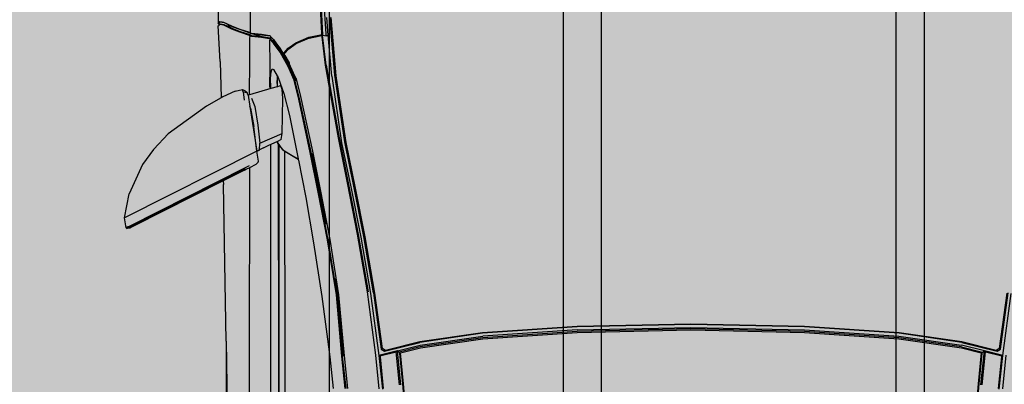
# Model space of a CAD drawing. Units: inches. Extents: x 1884 to 2398, y 474 to 1488.
# Tile 25 of 39: x 2275 to 2348, y 672 to 699. Entities that reach past the tile are written whole.
import ezdxf

# ---------------------------------------------------------------- set-up
doc = ezdxf.new("R2010")
doc.units = ezdxf.units.IN
doc.header["$MEASUREMENT"] = 0
doc.layers.get('0').update_dxf_attribs({"color": 250})
doc.layers.add('A-ANNO-DIMS', color=2, linetype='Continuous', lineweight=18)
doc.layers.add('C-VEHI', color=8, linetype='Continuous', lineweight=18)
doc.layers.add('Edges', color=250, linetype='Continuous')
doc.layers.add('L-PVMT-PATT', color=9, linetype='Continuous', lineweight=13, true_color=0xc7c8ca)
doc.styles.get("Standard").update_dxf_attribs({"font": 'arial.ttf'})
doc.dimstyles.get("Standard").update_dxf_attribs({"dimtxt": 7, "dimasz": 0.18, "dimexe": 0.18, "dimexo": 0.0625, "dimgap": 0.09, "dimtad": 0, "dimtih": 1, "dimtoh": 1, "dimzin": 0, "dimdsep": 46, "dimlunit": 3, "dimtxsty": 'Standard', "dimcen": 0.09, "dimadec": 0, "dimazin": 0, "dimtfac": 1, "dimtofl": 0, "dimtmove": 0, "dimatfit": 3, "dimfxl": 1, "dimtolj": 1, "dimtzin": 0, "dimarcsym": 0})

# ---------------------------------------------------------------- blocks, each defined once
blk = doc.blocks.new('Nissan Qashqai pl')
at = {"layer": 'Edges'}
for p, q in [((9.2669, 12.5088), (9.1605, 12.5233)), ((9.2789, 12.5131), (9.1617, 12.5292)), ((9.1612, 12.5208), (9.2656, 12.5065)), ((9.2543, 12.4356), (9.2707, 12.5028)), ((9.2656, 12.5065), (9.2669, 12.5088)), ((9.2656, 12.5065), (9.2694, 12.5006)), ((9.2707, 12.5028), (9.2669, 12.5088)), ((9.2707, 12.5028), (9.2694, 12.5006)), ((9.2789, 12.5131), (9.2704, 12.4783)), ((9.2724, 12.4804), (9.2799, 12.5114)), ((9.2783, 12.5191), (9.3422, 12.5126)), ((9.2799, 12.5114), (9.2789, 12.5131)), ((9.3427, 12.5066), (9.2789, 12.5131)), ((9.2819, 12.5112), (9.2799, 12.5114)), ((9.2803, 12.5116), (9.2822, 12.5118)), ((9.3418, 12.5051), (9.2819, 12.5112)), ((9.2694, 12.5006), (9.2535, 12.4354)), ((9.2704, 12.4783), (9.2598, 12.4348)), ((9.2629, 12.435), (9.2726, 12.4746)), ((9.2649, 12.4348), (9.2741, 12.4725)), ((9.2724, 12.4804), (9.2704, 12.4783)), ((9.2726, 12.4746), (9.2704, 12.4783)), ((9.3346, 12.4718), (9.2704, 12.4783)), ((9.3346, 12.4741), (9.2724, 12.4804)), ((9.2746, 12.4744), (9.2726, 12.4746)), ((9.2741, 12.4725), (9.3326, 12.4666)), ((9.333, 12.4685), (9.2746, 12.4744)), ((9.3326, 12.4666), (9.4, 12.4609)), ((9.4004, 12.4629), (9.333, 12.4685)), ((9.2535, 12.4354), (9.2362, 12.3167)), ((9.2543, 12.4356), (9.2371, 12.3169)), ((9.2426, 12.3164), (9.2598, 12.4348)), ((9.2629, 12.435), (9.2457, 12.3164)), ((9.2476, 12.3163), (9.2649, 12.4348)), ((9.2362, 12.3167), (9.2241, 12.1376)), ((9.2371, 12.3169), (9.2249, 12.1376)), ((9.2305, 12.1375), (9.2426, 12.3164)), ((9.2457, 12.3164), (9.2335, 12.1374)), ((9.2355, 12.1374), (9.2476, 12.3163)), ((9.2241, 12.1376), (9.2195, 11.9221)), ((9.2249, 12.1376), (9.2203, 11.9221)), ((9.2259, 11.9221), (9.2305, 12.1375)), ((9.2335, 12.1374), (9.2289, 11.9221)), ((9.2308, 11.9221), (9.2355, 12.1374)), ((9.2195, 11.9221), (9.2241, 11.7066)), ((9.2203, 11.9221), (9.2249, 11.7065)), ((9.2305, 11.7067), (9.2259, 11.9221)), ((9.2289, 11.9221), (9.2335, 11.7067)), ((9.2355, 11.7068), (9.2308, 11.9221)), ((9.2241, 11.7066), (9.2362, 11.5274)), ((9.2249, 11.7065), (9.2371, 11.5273)), ((9.2305, 11.7067), (9.2426, 11.5277)), ((9.2335, 11.7067), (9.2457, 11.5277)), ((9.2476, 11.5278), (9.2355, 11.7068)), ((9.2362, 11.5274), (9.2535, 11.4087)), ((9.2371, 11.5273), (9.2543, 11.4085)), ((9.2598, 11.4093), (9.2426, 11.5277)), ((9.2457, 11.5277), (9.2629, 11.4092)), ((9.2649, 11.4094), (9.2476, 11.5278)), ((9.2535, 11.4087), (9.2694, 11.3436)), ((9.2707, 11.3414), (9.2543, 11.4085)), ((9.2704, 11.3659), (9.2598, 11.4093)), ((9.2629, 11.4092), (9.2726, 11.3695)), ((9.2741, 11.3716), (9.2649, 11.4094)), ((9.4, 11.3832), (9.3326, 11.3776)), ((9.3346, 11.3724), (9.2704, 11.3659)), ((9.2704, 11.3659), (9.2726, 11.3695)), ((9.2704, 11.3659), (9.2724, 11.3637)), ((9.2704, 11.3659), (9.2789, 11.331)), ((9.3346, 11.37), (9.2724, 11.3637)), ((9.2726, 11.3695), (9.2746, 11.3697)), ((9.3326, 11.3776), (9.2741, 11.3716)), ((9.2746, 11.3697), (9.333, 11.3757)), ((9.333, 11.3757), (9.4004, 11.3813)), ((9.2799, 11.3328), (9.2724, 11.3637)), ((9.1605, 11.3208), (9.2669, 11.3354)), ((9.2656, 11.3376), (9.1612, 11.3233)), ((9.1617, 11.315), (9.2789, 11.331)), ((9.2694, 11.3436), (9.2656, 11.3376)), ((9.2669, 11.3354), (9.2656, 11.3376)), ((9.2669, 11.3354), (9.2707, 11.3414)), ((9.2694, 11.3436), (9.2707, 11.3414)), ((9.3422, 11.3316), (9.2783, 11.3251)), ((9.2789, 11.331), (9.3427, 11.3375)), ((9.2789, 11.331), (9.2799, 11.3327)), ((9.2799, 11.3328), (9.2819, 11.333)), ((9.2799, 11.3327), (9.2799, 11.3328)), ((9.2799, 11.3327), (9.2811, 11.3325)), ((9.2819, 11.333), (9.3418, 11.3391)), ((9.1584, 11.3091), (9.0495, 11.2906)), ((9.0497, 11.2918), (9.1586, 11.3104)), ((9.1605, 11.3208), (9.0538, 11.3023)), ((9.1612, 11.3233), (9.0546, 11.3048)), ((9.0552, 11.2965), (9.1617, 11.315)), ((9.2783, 11.3251), (9.1584, 11.3091)), ((9.0495, 11.2906), (8.9521, 11.2715)), ((8.9522, 11.2728), (9.0497, 11.2918)), ((9.0538, 11.3023), (8.9583, 11.2833)), ((9.0546, 11.3048), (8.9591, 11.2859)), ((8.9598, 11.2775), (9.0552, 11.2965)), ((8.8666, 11.2554), (8.9522, 11.2728)), ((8.9521, 11.2715), (8.8666, 11.2541)), ((8.9583, 11.2833), (8.8745, 11.266)), ((8.9591, 11.2859), (8.8754, 11.2687)), ((8.8761, 11.2602), (8.9598, 11.2775)), ((9.2801, 11.2648), (9.3418, 11.2713)), ((8.7287, 11.2307), (8.8666, 11.2554)), ((8.8666, 11.2541), (8.7292, 11.2295)), ((8.8745, 11.266), (8.7481, 11.2473)), ((8.8754, 11.2687), (8.7491, 11.2501)), ((8.7496, 11.2416), (8.8761, 11.2602)), ((9.0591, 11.2377), (9.1639, 11.2546)), ((9.133, 11.2481), (9.1647, 11.2532)), ((9.1639, 11.2546), (9.2801, 11.2648)), ((9.2803, 11.2606), (9.1644, 11.2503)), ((9.2804, 11.262), (9.1645, 11.2518)), ((9.1647, 11.2532), (9.1668, 11.2533)), ((9.2804, 11.2635), (9.1668, 11.2533)), ((9.3418, 11.2671), (9.2803, 11.2606)), ((9.3419, 11.2685), (9.2804, 11.262)), ((8.7481, 11.2473), (8.6375, 11.2376)), ((8.7491, 11.2501), (8.6386, 11.2404)), ((8.6721, 11.2348), (8.6387, 11.2319)), ((8.7496, 11.2416), (8.6721, 11.2348)), ((8.6721, 11.2348), (8.6733, 11.2313)), ((9.0601, 11.235), (8.8941, 11.2023)), ((8.9679, 11.2201), (9.0591, 11.2377)), ((9.06, 11.2335), (8.9696, 11.2157)), ((9.1644, 11.2503), (9.06, 11.2335)), ((9.1645, 11.2518), (9.0601, 11.235)), ((9.1676, 11.2229), (9.2814, 11.2377)), ((9.2814, 11.2377), (9.3416, 11.2442)), ((8.6683, 11.2226), (8.6197, 11.2201)), ((8.6203, 11.2213), (8.6721, 11.2241)), ((8.6699, 11.231), (8.622, 11.228)), ((8.671, 11.2227), (8.6683, 11.2226)), ((8.6721, 11.2312), (8.6699, 11.231)), ((8.6721, 11.2241), (8.671, 11.2227)), ((8.6716, 11.2199), (8.671, 11.2227)), ((8.6759, 11.1982), (8.6716, 11.2199)), ((8.6721, 11.2312), (8.6721, 11.2318)), ((8.6721, 11.2241), (8.6733, 11.2313)), ((8.6733, 11.2313), (8.6721, 11.2312)), ((8.7287, 11.2307), (8.6721, 11.2241)), ((8.6721, 11.2241), (8.6727, 11.2229)), ((8.6772, 11.1988), (8.6721, 11.2241)), ((8.6753, 11.2232), (8.6727, 11.2229)), ((8.6777, 11.1984), (8.6727, 11.2229)), ((8.7292, 11.2295), (8.6753, 11.2232)), ((8.8918, 11.205), (8.9679, 11.2201)), ((8.9696, 11.2157), (8.8942, 11.2009)), ((8.9318, 11.211), (8.9704, 11.2185)), ((8.9704, 11.2185), (8.9708, 11.2185)), ((8.9708, 11.2185), (9.03, 11.2304)), ((9.0656, 11.207), (9.1676, 11.2229)), ((8.6864, 11.1736), (8.6759, 11.1982)), ((8.6875, 11.1744), (8.6772, 11.1988)), ((8.6777, 11.1984), (8.6883, 11.1737)), ((8.7881, 11.1821), (8.8918, 11.205)), ((8.8941, 11.2023), (8.7925, 11.1802)), ((8.8942, 11.2009), (8.7931, 11.1789)), ((8.8961, 11.204), (8.9318, 11.211)), ((8.9797, 11.1924), (9.0656, 11.207)), ((8.7931, 11.1789), (8.7574, 11.1704)), ((8.7575, 11.1744), (8.7881, 11.1821)), ((8.7925, 11.1802), (8.7591, 11.1723)), ((8.8245, 11.1613), (8.9063, 11.1779)), ((8.9021, 11.1697), (8.9063, 11.1779)), ((8.9075, 11.1781), (8.9041, 11.1717)), ((8.9063, 11.1779), (8.9075, 11.1781)), ((8.9075, 11.1781), (8.9087, 11.1783)), ((8.9087, 11.1783), (8.9797, 11.1924)), ((8.697, 11.1592), (8.6864, 11.1736)), ((8.6979, 11.1603), (8.6875, 11.1744)), ((8.6883, 11.1737), (8.6987, 11.1597)), ((8.7055, 11.1514), (8.697, 11.1592)), ((8.6987, 11.1596), (8.6979, 11.1603)), ((8.6987, 11.1597), (8.6988, 11.1596)), ((8.6987, 11.1596), (8.6988, 11.1596)), ((8.6996, 11.1588), (8.6987, 11.1596)), ((8.6988, 11.1596), (8.6996, 11.1588)), ((8.6996, 11.1588), (8.6996, 11.1588)), ((8.6996, 11.1588), (8.7062, 11.1527)), ((8.7302, 11.1602), (8.7032, 11.145)), ((8.7312, 11.1591), (8.7042, 11.144)), ((8.7075, 11.1487), (8.7346, 11.1636)), ((8.7108, 11.1523), (8.7257, 11.1609)), ((8.7108, 11.1523), (8.7248, 11.1605)), ((8.7248, 11.1605), (8.7257, 11.1609)), ((8.7508, 11.1722), (8.7257, 11.1609)), ((8.7529, 11.17), (8.7302, 11.1602)), ((8.7574, 11.1704), (8.7312, 11.1591)), ((8.7346, 11.1636), (8.7577, 11.1732)), ((8.7346, 11.1636), (8.7491, 11.1703)), ((8.7491, 11.1703), (8.7576, 11.1743)), ((8.7508, 11.1722), (8.7491, 11.1703)), ((8.7532, 11.1733), (8.7508, 11.1722)), ((8.7529, 11.17), (8.7577, 11.1732)), ((8.757, 11.1718), (8.7529, 11.17)), ((8.7532, 11.1733), (8.7575, 11.1744)), ((8.7587, 11.1722), (8.757, 11.1718)), ((8.7575, 11.1744), (8.7576, 11.1743)), ((8.7576, 11.1743), (8.7582, 11.1734)), ((8.7577, 11.1732), (8.7582, 11.1734)), ((8.7582, 11.1734), (8.759, 11.1725)), ((8.759, 11.1725), (8.7587, 11.1722)), ((8.7591, 11.1723), (8.7587, 11.1722)), ((8.759, 11.1725), (8.7591, 11.1723)), ((8.7828, 11.1508), (8.8245, 11.1613)), ((8.8893, 11.1486), (8.9021, 11.1697)), ((8.9041, 11.1717), (8.8927, 11.1528)), ((8.7042, 11.144), (8.687, 11.131)), ((8.6884, 11.1371), (8.6973, 11.144)), ((8.6917, 11.1371), (8.7075, 11.1487)), ((8.7032, 11.145), (8.6927, 11.1371)), ((8.6973, 11.144), (8.698, 11.1446)), ((8.698, 11.1446), (8.6981, 11.1446)), ((8.7071, 11.15), (8.6981, 11.1446)), ((8.7062, 11.1527), (8.6996, 11.1588)), ((8.707, 11.15), (8.7055, 11.1514)), ((8.7067, 11.1522), (8.7062, 11.1527)), ((8.7083, 11.1508), (8.7067, 11.1522)), ((8.707, 11.15), (8.7083, 11.1508)), ((8.7071, 11.15), (8.707, 11.15)), ((8.707, 11.15), (8.707, 11.15)), ((8.7083, 11.1508), (8.7071, 11.15)), ((8.7083, 11.1507), (8.7102, 11.1519)), ((8.7083, 11.1508), (8.7083, 11.1507)), ((8.7102, 11.1519), (8.7108, 11.1523)), ((8.7492, 11.1383), (8.7524, 11.1401)), ((8.7524, 11.1401), (8.7828, 11.1508)), ((8.7748, 11.1475), (8.7678, 11.1453)), ((8.7678, 11.1453), (8.7698, 11.1385)), ((8.7916, 11.1488), (8.7748, 11.1475)), ((8.8259, 11.1483), (8.7916, 11.1488)), ((8.8585, 11.1473), (8.8259, 11.1483)), ((8.87, 11.1455), (8.8585, 11.1473)), ((8.8771, 11.1054), (8.8585, 11.1473)), ((8.87, 11.1455), (8.8734, 11.1385)), ((8.8893, 11.1486), (8.8751, 11.1387)), ((8.8768, 11.1385), (8.879, 11.1402)), ((8.879, 11.1402), (8.881, 11.1418)), ((8.879, 11.1402), (9.3198, 11.1403)), ((8.881, 11.1418), (8.8893, 11.1486)), ((9.3225, 11.1421), (8.881, 11.1418)), ((8.8913, 11.1506), (8.8893, 11.1486)), ((8.8927, 11.1528), (8.8913, 11.1506)), ((9.3225, 11.1531), (8.8927, 11.1528)), ((9.3198, 11.1403), (9.4922, 11.1409)), ((9.4936, 11.1538), (9.3225, 11.1531)), ((9.4936, 11.1428), (9.3225, 11.1421)), ((8.6703, 11.1081), (8.6727, 11.1235)), ((8.6714, 11.1088), (8.6737, 11.1245)), ((8.6727, 11.1235), (8.6737, 11.1245)), ((8.6737, 11.1245), (8.6746, 11.1253)), ((8.6805, 11.1309), (8.6746, 11.1253)), ((8.6746, 11.1253), (8.6785, 11.1253)), ((8.6777, 11.1246), (8.6755, 11.1099)), ((8.6788, 11.1237), (8.6764, 11.1083)), ((8.6785, 11.1253), (8.6777, 11.1246)), ((8.6815, 11.128), (8.6785, 11.1253)), ((8.687, 11.131), (8.6788, 11.1237)), ((8.6805, 11.1309), (8.6884, 11.1371)), ((8.6815, 11.128), (8.6818, 11.1288)), ((8.6817, 11.1282), (8.6815, 11.128)), ((8.6859, 11.132), (8.6817, 11.1282)), ((8.6817, 11.1282), (8.6818, 11.1288)), ((8.6818, 11.1288), (8.6902, 11.136)), ((8.6818, 11.1238), (8.7026, 11.1238)), ((8.6927, 11.1371), (8.6859, 11.132)), ((8.6884, 11.1371), (8.6917, 11.1371)), ((8.6902, 11.136), (8.6917, 11.1371)), ((8.6923, 11.1371), (8.6927, 11.1371)), ((8.7026, 11.1238), (8.7026, 11.1239)), ((8.7026, 11.1238), (8.7072, 11.1239)), ((8.7072, 11.1239), (8.7072, 11.1239)), ((8.7072, 11.1239), (8.7273, 11.1239)), ((8.7273, 11.1239), (8.7273, 11.124)), ((8.7273, 11.1239), (8.7354, 11.124)), ((8.7354, 11.1241), (8.7354, 11.124)), ((8.7354, 11.124), (8.742, 11.124)), ((8.7361, 11.1283), (8.7373, 11.1314)), ((8.7415, 11.1265), (8.7361, 11.1283)), ((8.7373, 11.1314), (8.7492, 11.1383)), ((8.7534, 11.1257), (8.7415, 11.1265)), ((8.742, 11.1241), (8.742, 11.124)), ((8.742, 11.124), (8.742, 11.1241)), ((8.742, 11.124), (8.742, 11.124)), ((8.742, 11.124), (8.7426, 11.124)), ((8.7426, 11.1241), (8.7426, 11.124)), ((8.7426, 11.124), (8.7433, 11.124)), ((8.7433, 11.1241), (8.7433, 11.124)), ((8.7433, 11.124), (8.7711, 11.1241)), ((8.7492, 11.1383), (8.7572, 11.1379)), ((8.7711, 11.1241), (8.7516, 11.1241)), ((8.7718, 11.126), (8.7534, 11.1257)), ((8.7572, 11.1379), (8.7698, 11.1383)), ((8.7698, 11.1385), (8.7583, 11.1382)), ((8.7698, 11.1385), (8.7698, 11.1383)), ((8.7698, 11.1383), (8.7733, 11.126)), ((8.7733, 11.126), (8.7718, 11.126)), ((8.7733, 11.126), (8.7849, 11.0859)), ((8.8734, 11.1385), (8.8793, 11.1261)), ((8.8734, 11.1385), (8.8768, 11.1385)), ((8.8751, 11.1387), (8.8768, 11.1385)), ((9.3194, 11.1262), (8.8793, 11.1261)), ((8.8793, 11.1261), (8.8815, 11.1214)), ((9.4919, 11.1269), (9.3194, 11.1262)), ((8.6684, 11.0892), (8.6703, 11.1081)), ((8.6697, 11.0922), (8.6714, 11.1088)), ((8.6698, 11.0925), (8.6755, 11.1099)), ((8.6754, 11.1089), (8.6735, 11.0898)), ((8.6764, 11.1082), (8.6744, 11.0891)), ((8.6755, 11.1099), (8.6754, 11.1089)), ((8.6764, 11.1082), (8.6764, 11.1083)), ((8.8429, 11.1016), (8.8771, 11.1054)), ((8.8895, 11.1048), (8.8771, 11.1054)), ((8.8815, 11.1214), (8.892, 11.0998)), ((8.8815, 11.1214), (8.8895, 11.1048)), ((8.8908, 11.1021), (8.8895, 11.1048)), ((8.8906, 11.1024), (8.8895, 11.1048)), ((8.9106, 11.1029), (8.892, 11.0998)), ((8.9131, 11.102), (8.9106, 11.1029)), ((8.5326, 11.0874), (8.6675, 11.0866)), ((8.6606, 11.0674), (8.6667, 11.0857)), ((8.6616, 11.0683), (8.6675, 11.0862)), ((8.6718, 11.0868), (8.6657, 11.0684)), ((8.6667, 11.0857), (8.6675, 11.0862)), ((8.6728, 11.0858), (8.6667, 11.0675)), ((8.6674, 11.0864), (8.6675, 11.0865)), ((8.6675, 11.0865), (8.6675, 11.0866)), ((8.6676, 11.0866), (8.6675, 11.0866)), ((8.6675, 11.0862), (8.6679, 11.0864)), ((8.6676, 11.0864), (8.6677, 11.0866)), ((8.6677, 11.0866), (8.6676, 11.0866)), ((8.6682, 11.0866), (8.6677, 11.0866)), ((8.6679, 11.0864), (8.6682, 11.0866)), ((8.6682, 11.087), (8.6684, 11.0888)), ((8.6692, 11.0876), (8.6682, 11.0866)), ((8.6682, 11.087), (8.6692, 11.0876)), ((8.6682, 11.0866), (8.6682, 11.087)), ((8.6684, 11.0888), (8.6684, 11.0892)), ((8.6684, 11.0888), (8.6685, 11.089)), ((8.6692, 11.0876), (8.6697, 11.0922)), ((8.6697, 11.0922), (8.6698, 11.0925)), ((8.6729, 11.0874), (8.6718, 11.0868)), ((8.674, 11.0864), (8.6728, 11.0858)), ((8.6733, 11.0875), (8.6729, 11.0874)), ((8.6735, 11.0898), (8.6733, 11.0875)), ((8.6742, 11.0866), (8.674, 11.0864)), ((8.6744, 11.0891), (8.6742, 11.0866)), ((8.6744, 11.0866), (8.6742, 11.0866)), ((8.6742, 11.0858), (8.6743, 11.086)), ((8.6744, 11.0864), (8.6744, 11.0866)), ((8.6773, 11.0865), (8.6744, 11.0866)), ((8.6791, 11.0864), (8.677, 11.0864)), ((8.6791, 11.0865), (8.6773, 11.0865)), ((8.6791, 11.0865), (8.6791, 11.0864)), ((8.6878, 11.0864), (8.6791, 11.0865)), ((8.7205, 11.0863), (8.6791, 11.0864)), ((8.6878, 11.0864), (8.6791, 11.0864)), ((8.6878, 11.0865), (8.6878, 11.0864)), ((8.6911, 11.0864), (8.6878, 11.0864)), ((8.7205, 11.0863), (8.6911, 11.0864)), ((8.7849, 11.0859), (8.7205, 11.0863)), ((8.7849, 11.0859), (8.7856, 11.0834)), ((8.7858, 11.0828), (8.807, 11.0862)), ((8.7917, 11.0895), (8.8075, 11.0955)), ((8.807, 11.0862), (8.8918, 11.0997)), ((8.8102, 11.0874), (8.807, 11.0862)), ((8.8075, 11.0955), (8.8429, 11.1016)), ((8.8102, 11.0874), (8.8455, 11.0936)), ((8.8918, 11.0997), (8.8455, 11.0936)), ((8.8906, 11.1024), (8.8911, 11.1013)), ((8.892, 11.0998), (8.8908, 11.1021)), ((8.8911, 11.1013), (8.8919, 11.0997)), ((8.8911, 11.1013), (8.8919, 11.0998)), ((8.8919, 11.0997), (8.8911, 11.1013)), ((8.8919, 11.0997), (8.8918, 11.0997)), ((8.8918, 11.0997), (9.0186, 10.8486)), ((8.892, 11.0998), (8.8919, 11.0998)), ((8.8919, 11.0998), (8.8919, 11.0997)), ((8.8919, 11.0997), (8.8919, 11.0997)), ((8.892, 11.0998), (8.892, 11.0998)), ((8.9171, 11.0978), (8.9131, 11.102)), ((8.9171, 11.0978), (8.917, 11.0974)), ((8.9171, 11.0978), (8.9233, 11.0855)), ((8.9232, 11.0779), (8.9194, 11.0854)), ((8.9233, 11.0855), (9.2886, 11.0848)), ((8.925, 11.0821), (8.9233, 11.0855)), ((9.2886, 11.0848), (9.4673, 11.0852)), ((8.6546, 11.0516), (8.6606, 11.0674)), ((8.6556, 11.0524), (8.6616, 11.0683)), ((8.6657, 11.0684), (8.6598, 11.0529)), ((8.6667, 11.0675), (8.6608, 11.0521)), ((8.7751, 11.0723), (8.7779, 11.0773)), ((8.7798, 11.0739), (8.7751, 11.0723)), ((8.7785, 11.0587), (8.7751, 11.0723)), ((8.7779, 11.0773), (8.7807, 11.0812)), ((8.7798, 11.0739), (8.7807, 11.0812)), ((8.7798, 11.0739), (8.7954, 11.0758)), ((8.7849, 11.0827), (8.7807, 11.0812)), ((8.7849, 11.0827), (8.7858, 11.0828)), ((8.7858, 11.0828), (8.7856, 11.0834)), ((9.0333, 10.8597), (8.9232, 11.0779)), ((8.928, 11.0762), (8.925, 11.0821)), ((9.0386, 10.8534), (8.9254, 11.0778)), ((8.928, 11.0762), (8.9483, 11.0359)), ((8.6472, 11.0366), (8.6546, 11.0516)), ((8.6482, 11.0375), (8.655, 11.0513)), ((8.6608, 11.0521), (8.6534, 11.0369)), ((8.6598, 11.0529), (8.655, 11.0432)), ((8.655, 11.0513), (8.6556, 11.0524)), ((8.655, 11.0513), (8.655, 11.0432)), ((8.7785, 11.0587), (8.7891, 11.0353)), ((8.646, 11.0289), (8.6468, 11.0337)), ((8.6489, 11.0263), (8.646, 11.0289)), ((8.6468, 11.0337), (8.6472, 11.0366)), ((8.647, 11.03), (8.6468, 11.0337)), ((8.647, 11.03), (8.6482, 11.0375)), ((8.6498, 11.0273), (8.647, 11.03)), ((8.6527, 11.0286), (8.6489, 11.0263)), ((8.6524, 11.0289), (8.6498, 11.0273)), ((8.6524, 11.0378), (8.651, 11.0302)), ((8.651, 11.0302), (8.652, 11.0292)), ((8.6534, 11.0369), (8.652, 11.0292)), ((8.652, 11.0292), (8.6524, 11.0289)), ((8.655, 11.0432), (8.6524, 11.0378)), ((8.6524, 11.0289), (8.6527, 11.0286)), ((8.6527, 11.0286), (8.6537, 11.0275)), ((8.7222, 11.0298), (8.6547, 11.0265)), ((8.7222, 11.0298), (8.7908, 11.0322)), ((8.7891, 11.0353), (8.7908, 11.0322)), ((8.7908, 11.0322), (8.8066, 11.0041)), ((8.9483, 11.0359), (8.9552, 11.0361)), ((8.9483, 11.0359), (9.0343, 10.8656)), ((9.2517, 11.0411), (8.9552, 11.0361)), ((9.2517, 11.0411), (9.5372, 11.0459)), ((9.2517, 11.0411), (9.351, 11.0411)), ((8.5838, 11.0251), (8.6489, 11.0263)), ((8.6547, 11.0265), (8.6537, 11.0275)), ((8.6537, 11.0275), (8.6537, 11.0275)), ((8.8066, 11.0041), (8.8591, 10.9315)), ((8.8591, 10.9315), (8.8879, 10.9041)), ((8.8885, 10.9037), (8.8879, 10.9041)), ((8.8885, 10.9037), (8.9173, 10.8831)), ((8.9173, 10.8831), (8.9731, 10.8577)), ((9.0343, 10.8656), (9.0347, 10.8648)), ((9.0347, 10.8648), (9.0362, 10.8619)), ((9.0362, 10.8619), (9.037, 10.8603)), ((9.0371, 10.8601), (9.037, 10.8603)), ((9.0186, 10.8486), (8.9731, 10.8577)), ((9.0374, 10.8517), (9.0186, 10.8486)), ((9.0356, 10.8553), (9.0333, 10.8597)), ((9.0356, 10.8553), (9.0374, 10.8517)), ((9.0371, 10.8601), (9.0376, 10.8591)), ((9.0376, 10.8591), (9.0371, 10.8595)), ((9.0386, 10.8534), (9.0374, 10.8517)), ((9.0376, 10.8591), (9.0386, 10.8534))]:
    blk.add_line(p, q, dxfattribs=at)
blk = doc.blocks.new('car')
blk.add_blockref('Nissan Qashqai pl', (-9.7433, -11.9151))
blk = doc.blocks.new('carr')
blk.add_blockref('car', (0.5124, -0.007))
blk = doc.blocks.new('*D23')
at = {"layer": 'A-ANNO-DIMS', "color": 0, "lineweight": -2, "transparency": 16777216}
for p, q in [((2272.304, 752.812), (2298.291, 752.812)), ((2298.111, 752.632), (2298.111, 670.29)), ((2298.111, 580.529), (2298.111, 662.871)), ((2272.304, 580.349), (2298.291, 580.349))]:
    blk.add_line(p, q, dxfattribs=at)
at = {"layer": 'A-ANNO-DIMS', "color": 0, "lineweight": 100, "transparency": 16777216}
for points in [[(2298.081, 752.632), (2298.141, 752.632), (2298.111, 752.812)], [(2298.081, 580.529), (2298.141, 580.529), (2298.111, 580.349)]]:
    blk.add_solid(points, dxfattribs=at)
at = {"layer": 'Defpoints', "color": 0, "lineweight": 100, "transparency": 16777216}
for p in [(2272.242, 752.812), (2272.242, 580.349), (2298.111, 580.349)]:
    blk.add_point(p, dxfattribs=at)
at = {"layer": 'A-ANNO-DIMS', "color": 0, "transparency": 16777216, "insert": (2298.111, 666.58), "char_height": 7, "attachment_point": 5}
blk.add_mtext('\\A1;CAR 14\'-4 1/2" TYP.', dxfattribs=at)
blk = doc.blocks.new('*D47')
at = {"layer": 'A-ANNO-DIMS', "color": 0, "lineweight": -2, "transparency": 16777216}
for p, q in [((2315.591, 959.704), (2315.591, 484.005)), ((2342.529, 959.704), (2342.529, 484.005)), ((2315.771, 484.185), (2319.606, 484.185)), ((2342.349, 484.185), (2338.513, 484.185))]:
    blk.add_line(p, q, dxfattribs=at)
at = {"layer": 'A-ANNO-DIMS', "color": 0, "lineweight": 100, "transparency": 16777216}
for points in [[(2315.771, 484.215), (2315.771, 484.155), (2315.591, 484.185)], [(2342.349, 484.215), (2342.349, 484.155), (2342.529, 484.185)]]:
    blk.add_solid(points, dxfattribs=at)
at = {"layer": 'Defpoints', "color": 0, "lineweight": 100, "transparency": 16777216}
for p in [(2315.591, 959.766), (2342.529, 959.766), (2342.529, 484.185)]:
    blk.add_point(p, dxfattribs=at)
at = {"layer": 'A-ANNO-DIMS', "color": 0, "transparency": 16777216, "insert": (2329.06, 484.185), "char_height": 7, "attachment_point": 5}
blk.add_mtext('\\A1;2\'-3"', dxfattribs=at)
blk = doc.blocks.new('*D49')
at = {"layer": 'A-ANNO-DIMS', "color": 0, "lineweight": -2, "transparency": 16777216}
for p, q in [((2318.409, 987.716), (2318.409, 484.005)), ((2340.409, 987.716), (2340.409, 484.005)), ((2318.589, 484.185), (2340.229, 484.185)), ((2340.409, 484.185), (2340.589, 484.185))]:
    blk.add_line(p, q, dxfattribs=at)
at = {"layer": 'A-ANNO-DIMS', "color": 0, "lineweight": 100, "transparency": 16777216}
for points in [[(2318.589, 484.215), (2318.589, 484.155), (2318.409, 484.185)], [(2340.229, 484.215), (2340.229, 484.155), (2340.409, 484.185)]]:
    blk.add_solid(points, dxfattribs=at)
at = {"layer": 'Defpoints', "color": 0, "lineweight": 100, "transparency": 16777216}
for p in [(2318.409, 987.778), (2340.409, 987.778), (2340.409, 484.185)]:
    blk.add_point(p, dxfattribs=at)
at = {"layer": 'A-ANNO-DIMS', "color": 0, "transparency": 16777216, "insert": (2352.373, 484.185), "char_height": 7, "attachment_point": 5}
blk.add_mtext('\\A1;1\'-10"', dxfattribs=at)

msp = doc.modelspace()

# ---------------------------------------------------------------- hatches: boundary and pattern name
at = {"layer": 'L-PVMT-PATT'}
h = msp.add_hatch(color=256, dxfattribs=at)
h.dxf.hatch_style = 1
h.paths.add_polyline_path([(2387.529, 769.966), (2351.529, 769.966), (2238.447, 769.966), (2238.447, 762.15), (2238.447, 754.445), (2126.529, 754.445), (2126.529, 676.183), (2134.868, 676.183), (2142.673, 676.183), (2142.673, 646.578), (2134.868, 646.578), (2126.529, 646.578), (2126.529, 640.17), (2387.529, 640.17)])
h.paths.add_polyline_path([(2387.529, 631.385), (2303.086, 631.385), (2303.086, 615.671), (2387.529, 615.671)])
h.paths.add_polyline_path([(2387.529, 640.17), (2126.529, 640.17), (2126.529, 631.385), (2387.529, 631.385)])
h.paths.add_polyline_path([(2393.529, 604.13), (2387.529, 604.13), (2387.529, 615.671), (2303.086, 615.671), (2303.086, 607.943), (2249.649, 607.943), (2126.529, 607.943), (2126.529, 533.885), (2393.529, 533.885)])
h.paths.add_polyline_path([(2257.825, 611.008), (2257.83, 611.337), (2257.915, 616.493), (2258.021, 621.805), (2258.146, 627.274), (2258.252, 631.385), (2126.529, 631.385), (2126.529, 611.008)])
h.paths.add_polyline_path([(2258.892, 611.285), (2258.888, 611.008), (2300.247, 611.008), (2300.247, 631.385), (2259.314, 631.385), (2259.206, 627.173), (2259.081, 621.72), (2258.976, 616.424)])

# ---------------------------------------------------------------- block references
at = {"layer": 'C-VEHI', "xscale": 39.37007874015748, "yscale": 39.37007874015748, "zscale": 39.37007874015748, "rotation": 270}
msp.add_blockref('carr', (2325.111, 676.232), dxfattribs=at)

# ---------------------------------------------------------------- dimensions: what is measured, and where the dimension line sits
at = {"layer": 'A-ANNO-DIMS'}
for base, p1, p2, picture, middle in [((2340.409, 484.185), (2318.409, 987.778), (2340.409, 987.778), '*D49', (2352.373, 484.185)), ((2342.529, 484.185), (2315.591, 959.766), (2342.529, 959.766), '*D47', (2329.06, 484.185))]:
    dim = msp.add_linear_dim(base=base, p1=p1, p2=p2, dimstyle='Standard', override={"dimdec": 1, "dimlfac": 1, "dimrnd": 0, "dimzin": 1, "dimdsep": 46, "dimlunit": 4, "dimfrac": 2}, dxfattribs=at)
    dim.commit()
    dim.dimension.update_dxf_attribs({"geometry": picture, "text_midpoint": middle})
dim = msp.add_linear_dim(base=(2298.111, 580.349), p1=(2272.242, 752.812), p2=(2272.242, 580.349), angle=270, text='CAR <> TYP.', dimstyle='Standard', override={"dimdec": 1, "dimlfac": 1, "dimrnd": 0, "dimzin": 1, "dimdsep": 46, "dimlunit": 4, "dimfrac": 2}, dxfattribs=at)
dim.commit()
dim.dimension.update_dxf_attribs({"geometry": '*D23', "text_midpoint": (2298.111, 666.58)})

doc.saveas('drawing.dxf')
